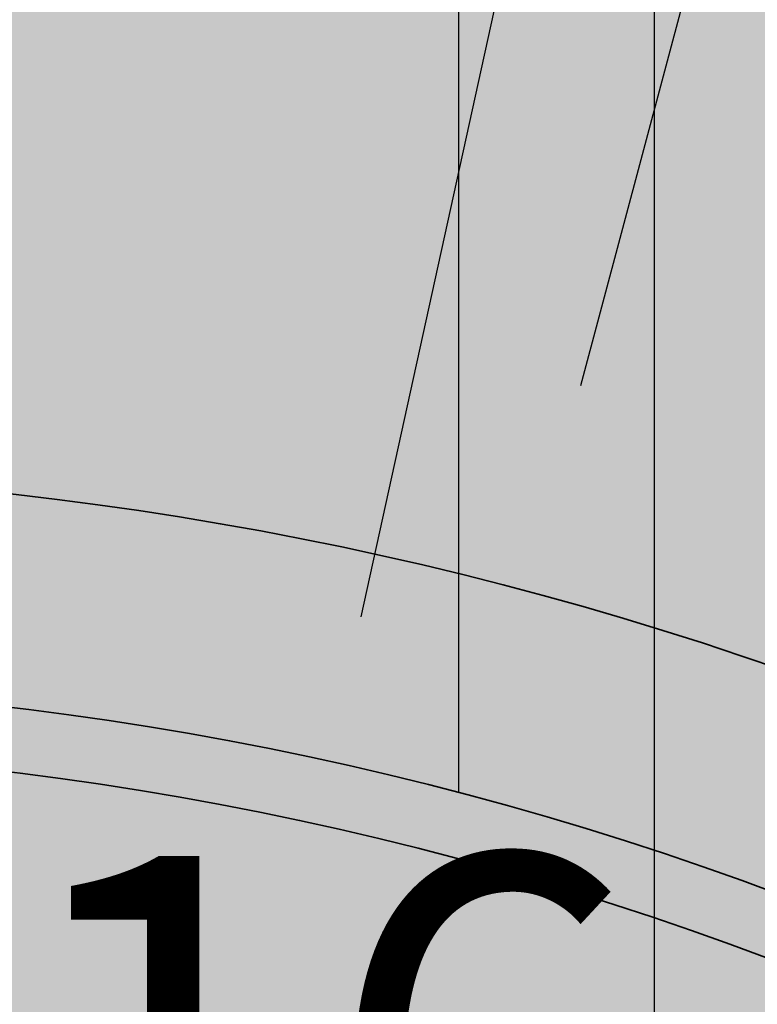
# Model space of a CAD drawing. Units: millimetres. Extents: x 130 to 1021, y 147 to 699.
# Tile 8 of 40: x 446 to 481, y 394 to 440. Entities that reach past the tile are written whole.
import ezdxf

# ---------------------------------------------------------------- set-up
doc = ezdxf.new("R2010")
doc.units = ezdxf.units.MM
doc.header["$MEASUREMENT"] = 0
for name, color, linetype, lineweight in [('A-ANNO-DIMS', 2, 'Continuous', 18), ('A-ELEV', 7, 'Continuous', 35), ('A-ELEV-PATT', 9, 'Continuous', 13)]:
    doc.layers.add(name, color=color, linetype=linetype, lineweight=lineweight)
doc.styles.get("Standard").update_dxf_attribs({"font": 'arial.ttf'})
doc.dimstyles.get("Standard").update_dxf_attribs({"dimtxt": 20, "dimasz": 10, "dimexe": 10, "dimexo": 10, "dimgap": 5, "dimtad": 0, "dimtih": 1, "dimtoh": 1, "dimdec": 0, "dimzin": 0, "dimdsep": 46, "dimtxsty": 'Standard', "dimcen": 5, "dimadec": 0, "dimazin": 0, "dimtfac": 1, "dimtdec": 0, "dimtofl": 0, "dimtmove": 0, "dimatfit": 3, "dimfxl": 1, "dimtolj": 1, "dimtzin": 0, "dimarcsym": 0})

# ---------------------------------------------------------------- blocks, each defined once
blk = doc.blocks.new('*D7')
at = {"layer": 'A-ANNO-DIMS', "color": 0, "lineweight": -2, "transparency": 16777216}
for p, q in [((399.374, 349.447), (413.374, 349.447)), ((423.374, 349.447), (433.374, 349.447)), ((389.374, 344.547), (389.374, 339.447)), ((423.374, 344.547), (423.374, 339.447))]:
    blk.add_line(p, q, dxfattribs=at)
at = {"layer": 'A-ANNO-DIMS', "color": 0, "transparency": 16777216}
for points in [[(399.374, 351.114), (399.374, 347.781), (389.374, 349.447)], [(413.374, 351.114), (413.374, 347.781), (423.374, 349.447)]]:
    blk.add_solid(points, dxfattribs=at)
at = {"layer": 'Defpoints', "color": 0, "transparency": 16777216}
for p in [(389.374, 354.547), (423.374, 354.547), (423.374, 349.447)]:
    blk.add_point(p, dxfattribs=at)
at = {"layer": 'A-ANNO-DIMS', "color": 0, "transparency": 16777216, "insert": (582.037, 349.447), "char_height": 20, "attachment_point": 5}
blk.add_mtext('\\A1;DOOR PANEL 34 TYP.', dxfattribs=at)
blk = doc.blocks.new('*D8')
at = {"layer": 'A-ANNO-DIMS', "color": 0, "lineweight": -2, "transparency": 16777216}
for p, q in [((428.474, 380.947), (428.474, 390.947)), ((428.474, 390.947), (438.474, 390.947)), ((433.374, 370.947), (438.474, 370.947)), ((433.374, 354.547), (438.474, 354.547)), ((428.474, 344.547), (428.474, 334.547))]:
    blk.add_line(p, q, dxfattribs=at)
at = {"layer": 'A-ANNO-DIMS', "color": 0, "transparency": 16777216}
for points in [[(426.807, 380.947), (430.14, 380.947), (428.474, 370.947)], [(426.807, 344.547), (430.14, 344.547), (428.474, 354.547)]]:
    blk.add_solid(points, dxfattribs=at)
at = {"layer": 'Defpoints', "color": 0, "transparency": 16777216}
for p in [(423.374, 370.947), (428.474, 370.947), (423.374, 354.547)]:
    blk.add_point(p, dxfattribs=at)
at = {"layer": 'A-ANNO-DIMS', "color": 0, "transparency": 16777216, "insert": (491.209, 390.947), "char_height": 20, "attachment_point": 5}
blk.add_mtext('\\A1;16 TYP.', dxfattribs=at)
blk = doc.blocks.new('*D11')
at = {"layer": 'A-ANNO-DIMS', "color": 0, "lineweight": -2, "transparency": 16777216}
for p, q in [((737.374, 648.699), (737.374, 149.739)), ((299.374, 566.947), (299.374, 149.739)), ((309.374, 159.739), (490.857, 159.739)), ((727.374, 159.739), (545.891, 159.739))]:
    blk.add_line(p, q, dxfattribs=at)
at = {"layer": 'A-ANNO-DIMS', "color": 0, "transparency": 16777216}
for points in [[(309.374, 161.406), (309.374, 158.073), (299.374, 159.739)], [(727.374, 161.406), (727.374, 158.073), (737.374, 159.739)]]:
    blk.add_solid(points, dxfattribs=at)
at = {"layer": 'Defpoints', "color": 0, "transparency": 16777216}
for p in [(737.374, 658.699), (299.374, 576.947), (737.374, 159.739)]:
    blk.add_point(p, dxfattribs=at)
at = {"layer": 'A-ANNO-DIMS', "color": 0, "transparency": 16777216, "insert": (518.374, 159.739), "char_height": 20, "attachment_point": 5}
blk.add_mtext('\\A1;438', dxfattribs=at)
blk = doc.blocks.new('*D12')
at = {"layer": 'A-ANNO-DIMS', "color": 0, "lineweight": -2, "transparency": 16777216}
for p, q in [((477.374, 661.947), (265.074, 661.947)), ((275.074, 651.947), (275.074, 438.205)), ((275.074, 194.039), (275.074, 407.782)), ((357.163, 184.039), (265.074, 184.039))]:
    blk.add_line(p, q, dxfattribs=at)
at = {"layer": 'A-ANNO-DIMS', "color": 0, "transparency": 16777216}
for points in [[(273.407, 651.947), (276.74, 651.947), (275.074, 661.947)], [(273.407, 194.039), (276.74, 194.039), (275.074, 184.039)]]:
    blk.add_solid(points, dxfattribs=at)
at = {"layer": 'Defpoints', "color": 0, "transparency": 16777216}
for p in [(275.074, 661.947), (487.374, 661.947), (367.163, 184.039)]:
    blk.add_point(p, dxfattribs=at)
at = {"layer": 'A-ANNO-DIMS', "color": 0, "transparency": 16777216, "insert": (275.074, 422.993), "char_height": 20, "attachment_point": 5}
blk.add_mtext('\\A1;477.9', dxfattribs=at)
blk = doc.blocks.new('*D16')
at = {"layer": 'A-ANNO-DIMS', "color": 0, "lineweight": -2, "transparency": 16777216}
for p, q in [((357.941, 411.947), (357.941, 696.247)), ((363.922, 579.884), (363.922, 696.247)), ((347.941, 686.247), (337.941, 686.247)), ((373.922, 686.247), (383.922, 686.247))]:
    blk.add_line(p, q, dxfattribs=at)
at = {"layer": 'A-ANNO-DIMS', "color": 0, "transparency": 16777216}
for points in [[(347.941, 687.914), (347.941, 684.581), (357.941, 686.247)], [(373.922, 687.914), (373.922, 684.581), (363.922, 686.247)]]:
    blk.add_solid(points, dxfattribs=at)
at = {"layer": 'Defpoints', "color": 0, "transparency": 16777216}
for p in [(363.922, 686.247), (363.922, 569.884), (357.941, 401.947)]:
    blk.add_point(p, dxfattribs=at)
at = {"layer": 'A-ANNO-DIMS', "color": 0, "transparency": 16777216, "insert": (420.737, 686.247), "char_height": 20, "attachment_point": 5}
blk.add_mtext('\\A1;5.981', dxfattribs=at)
blk = doc.blocks.new('*D18')
at = {"layer": 'A-ANNO-DIMS', "color": 0, "lineweight": -2, "transparency": 16777216}
for p, q in [((375.85, 490.216), (375.85, 696.247)), ((382.374, 388.947), (382.374, 696.247)), ((365.85, 686.247), (355.85, 686.247)), ((392.374, 686.247), (402.374, 686.247))]:
    blk.add_line(p, q, dxfattribs=at)
at = {"layer": 'A-ANNO-DIMS', "color": 0, "transparency": 16777216}
for points in [[(365.85, 687.914), (365.85, 684.581), (375.85, 686.247)], [(392.374, 687.914), (392.374, 684.581), (382.374, 686.247)]]:
    blk.add_solid(points, dxfattribs=at)
at = {"layer": 'Defpoints', "color": 0, "transparency": 16777216}
for p in [(382.374, 686.247), (375.85, 480.216), (382.374, 378.947)]:
    blk.add_point(p, dxfattribs=at)
at = {"layer": 'A-ANNO-DIMS', "color": 0, "transparency": 16777216, "insert": (441.132, 686.247), "char_height": 20, "attachment_point": 5}
blk.add_mtext('\\A1;6.524', dxfattribs=at)
blk = doc.blocks.new('*D19')
at = {"layer": 'A-ANNO-DIMS', "color": 0, "lineweight": -2, "transparency": 16777216}
for p, q in [((382.374, 388.947), (382.374, 696.247)), ((414.652, 510.881), (414.652, 696.247)), ((392.374, 686.247), (404.652, 686.247)), ((414.652, 686.247), (424.652, 686.247))]:
    blk.add_line(p, q, dxfattribs=at)
at = {"layer": 'A-ANNO-DIMS', "color": 0, "transparency": 16777216}
for points in [[(392.374, 687.914), (392.374, 684.581), (382.374, 686.247)], [(404.652, 687.914), (404.652, 684.581), (414.652, 686.247)]]:
    blk.add_solid(points, dxfattribs=at)
at = {"layer": 'Defpoints', "color": 0, "transparency": 16777216}
for p in [(414.652, 686.247), (414.652, 500.881), (382.374, 378.947)]:
    blk.add_point(p, dxfattribs=at)
at = {"layer": 'A-ANNO-DIMS', "color": 0, "transparency": 16777216, "insert": (463.411, 686.247), "char_height": 20, "attachment_point": 5}
blk.add_mtext('\\A1;32.28', dxfattribs=at)
blk = doc.blocks.new('*D20')
at = {"layer": 'A-ANNO-DIMS', "color": 0, "lineweight": -2, "transparency": 16777216}
for p, q in [((414.652, 510.881), (414.652, 696.247)), ((432.374, 388.947), (432.374, 696.247)), ((404.652, 686.247), (394.652, 686.247)), ((442.374, 686.247), (452.374, 686.247))]:
    blk.add_line(p, q, dxfattribs=at)
at = {"layer": 'A-ANNO-DIMS', "color": 0, "transparency": 16777216}
for points in [[(404.652, 687.914), (404.652, 684.581), (414.652, 686.247)], [(442.374, 687.914), (442.374, 684.581), (432.374, 686.247)]]:
    blk.add_solid(points, dxfattribs=at)
at = {"layer": 'Defpoints', "color": 0, "transparency": 16777216}
for p in [(432.374, 686.247), (414.652, 500.881), (432.374, 378.947)]:
    blk.add_point(p, dxfattribs=at)
at = {"layer": 'A-ANNO-DIMS', "color": 0, "transparency": 16777216, "insert": (490.075, 686.247), "char_height": 20, "attachment_point": 5}
blk.add_mtext('\\A1;17.72', dxfattribs=at)
blk = doc.blocks.new('*D21')
at = {"layer": 'A-ANNO-DIMS', "color": 0, "lineweight": -2, "transparency": 16777216}
for p, q in [((432.374, 388.947), (432.374, 696.247)), ((447.374, 656.947), (447.374, 696.247)), ((422.374, 686.247), (412.374, 686.247)), ((457.374, 686.247), (467.374, 686.247))]:
    blk.add_line(p, q, dxfattribs=at)
at = {"layer": 'A-ANNO-DIMS', "color": 0, "transparency": 16777216}
for points in [[(422.374, 687.914), (422.374, 684.581), (432.374, 686.247)], [(457.374, 687.914), (457.374, 684.581), (447.374, 686.247)]]:
    blk.add_solid(points, dxfattribs=at)
at = {"layer": 'Defpoints', "color": 0, "transparency": 16777216}
for p in [(447.374, 686.247), (447.374, 646.947), (432.374, 378.947)]:
    blk.add_point(p, dxfattribs=at)
at = {"layer": 'A-ANNO-DIMS', "color": 0, "transparency": 16777216, "insert": (485.832, 686.247), "char_height": 20, "attachment_point": 5}
blk.add_mtext('\\A1;15', dxfattribs=at)
blk = doc.blocks.new('*D22')
at = {"layer": 'A-ANNO-DIMS', "color": 0, "lineweight": -2, "transparency": 16777216}
for p, q in [((447.374, 656.947), (447.374, 696.247)), ((466.767, 403.947), (466.767, 696.247)), ((437.374, 686.247), (427.374, 686.247)), ((476.767, 686.247), (486.767, 686.247))]:
    blk.add_line(p, q, dxfattribs=at)
at = {"layer": 'A-ANNO-DIMS', "color": 0, "transparency": 16777216}
for points in [[(437.374, 687.914), (437.374, 684.581), (447.374, 686.247)], [(476.767, 687.914), (476.767, 684.581), (466.767, 686.247)]]:
    blk.add_solid(points, dxfattribs=at)
at = {"layer": 'Defpoints', "color": 0, "transparency": 16777216}
for p in [(466.767, 686.247), (447.374, 646.947), (466.767, 393.947)]:
    blk.add_point(p, dxfattribs=at)
at = {"layer": 'A-ANNO-DIMS', "color": 0, "transparency": 16777216, "insert": (532.34, 686.247), "char_height": 20, "attachment_point": 5}
blk.add_mtext('\\A1;19.393', dxfattribs=at)
blk = doc.blocks.new('*D23')
at = {"layer": 'A-ANNO-DIMS', "color": 0, "lineweight": -2, "transparency": 16777216}
for p, q in [((466.767, 403.947), (466.767, 696.247)), ((475.988, 209.039), (475.988, 696.247)), ((456.767, 686.247), (446.767, 686.247)), ((485.988, 686.247), (495.988, 686.247))]:
    blk.add_line(p, q, dxfattribs=at)
at = {"layer": 'A-ANNO-DIMS', "color": 0, "transparency": 16777216}
for points in [[(456.767, 687.914), (456.767, 684.581), (466.767, 686.247)], [(485.988, 687.914), (485.988, 684.581), (475.988, 686.247)]]:
    blk.add_solid(points, dxfattribs=at)
at = {"layer": 'Defpoints', "color": 0, "transparency": 16777216}
for p in [(475.988, 686.247), (466.767, 393.947), (475.988, 199.039)]:
    blk.add_point(p, dxfattribs=at)
at = {"layer": 'A-ANNO-DIMS', "color": 0, "transparency": 16777216, "insert": (534.631, 686.247), "char_height": 20, "attachment_point": 5}
blk.add_mtext('\\A1;9.222', dxfattribs=at)
blk = doc.blocks.new('*D24')
at = {"layer": 'A-ANNO-DIMS', "color": 0, "lineweight": -2, "transparency": 16777216}
for p, q in [((475.988, 209.039), (475.988, 696.247)), ((487.374, 671.947), (487.374, 696.247)), ((465.988, 686.247), (455.988, 686.247)), ((497.374, 686.247), (507.374, 686.247))]:
    blk.add_line(p, q, dxfattribs=at)
at = {"layer": 'A-ANNO-DIMS', "color": 0, "transparency": 16777216}
for points in [[(465.988, 687.914), (465.988, 684.581), (475.988, 686.247)], [(497.374, 687.914), (497.374, 684.581), (487.374, 686.247)]]:
    blk.add_solid(points, dxfattribs=at)
at = {"layer": 'Defpoints', "color": 0, "transparency": 16777216}
for p in [(487.374, 686.247), (487.374, 661.947), (475.988, 199.039)]:
    blk.add_point(p, dxfattribs=at)
at = {"layer": 'A-ANNO-DIMS', "color": 0, "transparency": 16777216, "insert": (553.022, 686.247), "char_height": 20, "attachment_point": 5}
blk.add_mtext('\\A1;11.385', dxfattribs=at)
blk = doc.blocks.new('*D64')
at = {"layer": 'A-ANNO-DIMS', "color": 0, "lineweight": -2, "transparency": 16777216}
for p, q in [((502.049, 450.926), (502.049, 460.926)), ((497.049, 455.926), (507.049, 455.926)), ((363.96, 263.061), (409.922, 327.255)), ((353.96, 263.061), (363.96, 263.061))]:
    blk.add_line(p, q, dxfattribs=at)
at = {"layer": 'A-ANNO-DIMS', "color": 0, "transparency": 16777216}
blk.add_solid([(408.567, 328.225), (411.277, 326.284), (415.743, 335.385)], dxfattribs=at)
at = {"layer": 'Defpoints', "color": 0, "transparency": 16777216}
for p in [(502.049, 455.926), (415.743, 335.385)]:
    blk.add_point(p, dxfattribs=at)
at = {"layer": 'A-ANNO-DIMS', "color": 0, "transparency": 16777216, "insert": (297.8, 263.061), "char_height": 20, "attachment_point": 5}
blk.add_mtext('\\A1;R148.25', dxfattribs=at)
blk = doc.blocks.new('*D65')
at = {"layer": 'A-ANNO-DIMS', "color": 0, "lineweight": -2, "transparency": 16777216}
for p, q in [((495.463, 509.127), (472.508, 423.108)), ((505.463, 509.127), (495.463, 509.127)), ((427.374, 248.979), (427.374, 258.979)), ((422.374, 253.979), (432.374, 253.979))]:
    blk.add_line(p, q, dxfattribs=at)
at = {"layer": 'A-ANNO-DIMS', "color": 0, "transparency": 16777216}
blk.add_solid([(470.898, 423.538), (474.118, 422.679), (469.93, 413.447)], dxfattribs=at)
at = {"layer": 'Defpoints', "color": 0, "transparency": 16777216}
for p in [(469.93, 413.447), (427.374, 253.979)]:
    blk.add_point(p, dxfattribs=at)
at = {"layer": 'A-ANNO-DIMS', "color": 0, "transparency": 16777216, "insert": (561.623, 509.127), "char_height": 20, "attachment_point": 5}
blk.add_mtext('\\A1;R165.05', dxfattribs=at)
blk = doc.blocks.new('*D67')
at = {"layer": 'A-ANNO-DIMS', "color": 0, "lineweight": -2, "transparency": 16777216}
for p, q in [((479.756, 492.431), (462.144, 412.223)), ((489.756, 492.431), (479.756, 492.431)), ((427.07, 247.496), (427.07, 257.496)), ((422.07, 252.496), (432.07, 252.496))]:
    blk.add_line(p, q, dxfattribs=at)
at = {"layer": 'A-ANNO-DIMS', "color": 0, "transparency": 16777216}
blk.add_solid([(460.516, 412.58), (463.772, 411.865), (459.999, 402.455)], dxfattribs=at)
at = {"layer": 'Defpoints', "color": 0, "transparency": 16777216}
for p in [(459.999, 402.455), (427.07, 252.496)]:
    blk.add_point(p, dxfattribs=at)
at = {"layer": 'A-ANNO-DIMS', "color": 0, "transparency": 16777216, "insert": (545.841, 492.431), "char_height": 20, "attachment_point": 5}
blk.add_mtext('\\A1;R153.53', dxfattribs=at)
blk = doc.blocks.new('*D69')
at = {"layer": 'A-ANNO-DIMS', "color": 0, "lineweight": -2, "transparency": 16777216}
for p, q in [((507.746, 572.261), (483.091, 501.813)), ((517.746, 572.261), (507.746, 572.261)), ((433.191, 354.23), (433.191, 364.23)), ((428.191, 359.23), (438.191, 359.23))]:
    blk.add_line(p, q, dxfattribs=at)
at = {"layer": 'A-ANNO-DIMS', "color": 0, "transparency": 16777216}
blk.add_solid([(481.518, 502.363), (484.664, 501.262), (479.788, 492.374)], dxfattribs=at)
at = {"layer": 'Defpoints', "color": 0, "transparency": 16777216}
for p in [(479.788, 492.374), (433.191, 359.23)]:
    blk.add_point(p, dxfattribs=at)
at = {"layer": 'A-ANNO-DIMS', "color": 0, "transparency": 16777216, "insert": (573.824, 572.261), "char_height": 20, "attachment_point": 5}
blk.add_mtext('\\A1;R141.06', dxfattribs=at)
blk = doc.blocks.new('*D71')
at = {"layer": 'A-ANNO-DIMS', "color": 0, "lineweight": -2, "transparency": 16777216}
for p, q in [((492.108, 581.609), (472.542, 512.666)), ((502.108, 581.609), (492.108, 581.609)), ((432.65, 367.109), (432.65, 377.109)), ((427.65, 372.109), (437.65, 372.109))]:
    blk.add_line(p, q, dxfattribs=at)
at = {"layer": 'A-ANNO-DIMS', "color": 0, "transparency": 16777216}
blk.add_solid([(470.938, 513.121), (474.145, 512.211), (469.812, 503.046)], dxfattribs=at)
at = {"layer": 'Defpoints', "color": 0, "transparency": 16777216}
for p in [(469.812, 503.046), (432.65, 372.109)]:
    blk.add_point(p, dxfattribs=at)
at = {"layer": 'A-ANNO-DIMS', "color": 0, "transparency": 16777216, "insert": (548.493, 581.609), "char_height": 20, "attachment_point": 5}
blk.add_mtext('\\A1;R136.1', dxfattribs=at)
blk = doc.blocks.new('*D72')
at = {"layer": 'A-ANNO-DIMS', "color": 0, "lineweight": -2, "transparency": 16777216}
for p, q in [((460.658, 573.64), (451.279, 503.49)), ((470.658, 573.64), (460.658, 573.64)), ((432.115, 355.142), (432.115, 365.142)), ((427.115, 360.142), (437.115, 360.142))]:
    blk.add_line(p, q, dxfattribs=at)
at = {"layer": 'A-ANNO-DIMS', "color": 0, "transparency": 16777216}
blk.add_solid([(449.628, 503.711), (452.931, 503.27), (449.954, 493.579)], dxfattribs=at)
at = {"layer": 'Defpoints', "color": 0, "transparency": 16777216}
for p in [(449.954, 493.579), (432.115, 360.142)]:
    blk.add_point(p, dxfattribs=at)
at = {"layer": 'A-ANNO-DIMS', "color": 0, "transparency": 16777216, "insert": (526.64, 573.64), "char_height": 20, "attachment_point": 5}
blk.add_mtext('\\A1;R134.62', dxfattribs=at)

msp = doc.modelspace()

# ---------------------------------------------------------------- hatches: boundary and pattern name
at = {"layer": 'A-ELEV-PATT'}
h = msp.add_hatch(color=256, dxfattribs=at)
h.dxf.hatch_style = 1
h.paths.add_polyline_path([(737.3738, 658.6988, 0.0135961), (632.4019, 661.9473), (607.3738, 661.9473), (487.3738, 661.9473), (487.3738, 649.9473), (607.3738, 649.9473), (632.3794, 649.9473, -0.0136841), (737.3738, 646.6784)])
h.paths.add_polyline_path([(732.3738, 643.9599, 0.0130529), (632.3738, 646.9473), (607.3738, 646.9473), (487.3738, 646.9473), (487.3738, 596.9473), (632.3738, 596.9473, -0.0130529), (732.3738, 593.9599)])
h.paths.add_polyline_path([(737.3738, 593.6732, 0.0137063), (632.3738, 596.9473), (487.3738, 596.9473), (487.3738, 586.9473), (632.355, 586.9473, -0.0137808), (737.3738, 583.6559)])
h.paths.add_polyline_path([(447.3738, 646.9473), (307.3738, 646.9473), (302.3738, 646.9473), (302.3738, 634.9473), (447.3738, 634.9473)])
h.paths.add_polyline_path([(447.3738, 631.9473), (307.3738, 631.9473), (307.3738, 586.9473), (447.3738, 586.9473)])
h.paths.add_polyline_path([(447.3738, 586.9473), (307.3738, 586.9473), (302.3738, 586.9473), (302.3738, 576.9473), (447.3738, 576.9473)])
h.paths.add_polyline_path([(447.3738, 573.9473), (367.3738, 573.9473), (367.3738, 539.9473), (447.3738, 539.9473)])
h.paths.add_polyline_path([(447.3738, 537.9473), (367.3738, 537.9473), (367.3738, 507.9473), (400.392, 507.4253, -0.001728), (401.3281, 507.6451, -0.5220025), (425.6117, 511.0391, -0.0391849), (447.3738, 510.4359), (447.3738, 510.7883)])
h.paths.add_polyline_path([(394.7238, 505.9473), (367.3738, 505.9473), (367.3738, 476.9473, -0.0146512), (375.8501, 480.2159), (376.1506, 499.2266, -0.0355419)])
h.paths.add_polyline_path([(632.3738, 583.9473), (552.3738, 583.9473), (552.3738, 550.9473), (632.3738, 550.9473)])
h.paths.add_polyline_path([(632.3738, 548.9473), (552.3738, 548.9473), (552.3738, 515.9473), (632.3738, 515.9473)])
h.paths.add_polyline_path([(632.3738, 513.9473), (552.3738, 513.9473), (552.3738, 476.9473), (632.3738, 476.9473)])
h.paths.add_polyline_path([(737.3738, 473.6903, 0.0136326), (632.3926, 476.9473), (552.3738, 476.9473), (487.3738, 476.9473), (487.3738, 466.9473), (632.3738, 466.9473, -0.0137063), (737.3738, 463.6732)])
h.paths.add_polyline_path([(732.3738, 460.9552, 0.0130741), (632.3681, 463.9473), (487.3738, 463.9473), (487.3738, 407.735, -0.0032286), (489.3544, 406.9473), (632.3926, 406.9473, -0.0129826), (732.3738, 403.9755)])
h.paths.add_polyline_path([(487.3738, 463.9473, 0.20133), (367.3738, 463.9473), (367.3738, 407.735, -0.1882031), (487.3738, 407.735)])
h.paths.add_polyline_path([(367.3738, 476.9473), (367.3738, 466.9473, -0.2013309), (487.3738, 466.9473), (487.3738, 476.9473, 0.20133)])
h.paths.add_polyline_path([(367.3738, 463.9473), (307.3738, 463.9473), (307.3738, 401.9473), (357.9413, 401.9473), (367.3738, 407.735)])
h.paths.add_polyline_path([(367.3738, 476.9473), (302.3738, 476.9473), (302.3738, 466.9473), (367.3738, 466.9473)])
h.paths.add_polyline_path([(632.8184, 366.9453), (552.3738, 366.9453), (552.3738, 393.9473), (632.8184, 393.9473)])
h.paths.add_polyline_path([(632.8184, 357.2114), (632.8184, 363.9453), (552.3738, 363.9453), (552.3738, 357.2114), (552.3738, 336.9453), (632.8184, 336.9453)])
h.paths.add_polyline_path([(632.8184, 333.9453), (552.3738, 333.9453), (552.3738, 306.9453), (632.8184, 306.9453)])
h.paths.add_polyline_path([(632.8184, 303.9453), (552.3738, 303.9453), (552.3738, 273.9473), (632.355, 273.9473, 0.0000608), (632.8184, 273.9491)])
h.paths.add_polyline_path([(737.3738, 403.6903, 0.0136326), (632.3926, 406.9473), (489.3544, 406.9473, 0.1915481), (367.3738, 407.735), (367.3738, 396.9473, -0.2013309), (487.3738, 396.9473), (632.3738, 396.9473, -0.0137063), (737.3738, 393.6732)])
h.paths.add_polyline_path([(357.9413, 401.9473), (307.3738, 401.9473), (307.3738, 391.9473), (357.9413, 391.9473)])
h.paths.add_polyline_path([(357.9413, 357.2114), (357.9413, 388.9473), (307.3738, 388.9473), (307.3738, 357.2114), (307.3738, 273.9473), (357.9413, 273.9473)])
h.paths.add_polyline_path([(732.3738, 263.93, -0.0130317), (632.3794, 260.9473), (466.7667, 260.9473), (466.7667, 240.9473), (469.8406, 236.978), (469.8406, 221.978), (472.9145, 218.0087), (472.9145, 213.9473), (607.3738, 213.9473), (732.3738, 213.9473)])
h.paths.add_polyline_path([(732.3738, 290.889), (722.479, 290.889), (722.479, 301.889), (732.3738, 301.889), (732.3738, 305.889), (722.479, 305.889), (722.479, 316.889), (732.3738, 316.889), (732.3738, 320.889), (722.479, 320.889), (722.479, 331.889), (732.3738, 331.889), (732.3738, 335.889), (722.479, 335.889), (722.479, 346.889), (732.3738, 346.889), (732.3738, 350.889), (722.479, 350.889), (722.479, 361.889), (732.3738, 361.889), (732.3738, 365.889), (722.479, 365.889), (722.479, 376.889), (732.3738, 376.889), (732.3738, 380.889), (722.479, 380.889), (722.479, 391.4848, 0.0005233), (718.479, 391.6843), (718.479, 380.889), (707.479, 380.889), (707.479, 392.1896, 0.0005231), (703.479, 392.3576), (703.479, 380.889), (692.479, 380.889), (692.479, 392.7765, 0.0005229), (688.479, 392.9131), (688.479, 380.889), (677.479, 380.889), (677.479, 393.2456, 0.0005228), (673.479, 393.3508), (673.479, 380.889), (662.479, 380.889), (662.479, 393.597, 0.0005227), (658.479, 393.6709), (658.479, 380.889), (647.479, 380.889), (647.479, 393.8308, 0.0005226), (643.479, 393.8732), (643.479, 380.889), (632.8184, 380.889), (632.8184, 376.889), (643.479, 376.889), (643.479, 365.889), (632.8184, 365.889), (632.8184, 361.889), (643.479, 361.889), (643.479, 350.889), (632.8184, 350.889), (632.8184, 346.889), (643.479, 346.889), (643.479, 335.889), (632.8184, 335.889), (632.8184, 331.889), (643.479, 331.889), (643.479, 320.889), (632.8184, 320.889), (632.8184, 316.889), (643.479, 316.889), (643.479, 305.889), (632.8184, 305.889), (632.8184, 301.889), (643.479, 301.889), (643.479, 290.889), (632.8184, 290.889), (632.8184, 286.889), (643.479, 286.889), (643.479, 274.0217, 0.0005246), (647.479, 274.0643), (647.479, 286.889), (658.479, 286.889), (658.479, 274.2248, 0.0005246), (662.479, 274.2989), (662.479, 286.889), (673.479, 286.889), (673.479, 274.546, 0.0005247), (677.479, 274.6516), (677.479, 286.889), (688.479, 286.889), (688.479, 274.9853, 0.0005248), (692.479, 275.1224), (692.479, 286.889), (703.479, 286.889), (703.479, 275.5429, 0.000525), (707.479, 275.7115), (707.479, 286.889), (718.479, 286.889), (718.479, 276.2187, 0.0005252), (722.479, 276.4189), (722.479, 286.889), (732.3738, 286.889)])
h.paths.add_polyline_path([(718.479, 290.889), (707.479, 290.889), (707.479, 301.889), (718.479, 301.889)], flags=16)
h.paths.add_polyline_path([(703.479, 290.889), (692.479, 290.889), (692.479, 301.889), (703.479, 301.889)], flags=16)
h.paths.add_polyline_path([(718.479, 305.889), (707.479, 305.889), (707.479, 316.889), (718.479, 316.889)], flags=16)
h.paths.add_polyline_path([(703.479, 305.889), (692.479, 305.889), (692.479, 316.889), (703.479, 316.889)], flags=16)
h.paths.add_polyline_path([(688.479, 290.889), (677.479, 290.889), (677.479, 301.889), (688.479, 301.889)], flags=16)
h.paths.add_polyline_path([(718.479, 320.889), (707.479, 320.889), (707.479, 331.889), (718.479, 331.889)], flags=16)
h.paths.add_polyline_path([(688.479, 305.889), (677.479, 305.889), (677.479, 316.889), (688.479, 316.889)], flags=16)
h.paths.add_polyline_path([(703.479, 320.889), (692.479, 320.889), (692.479, 331.889), (703.479, 331.889)], flags=16)
h.paths.add_polyline_path([(688.479, 320.889), (677.479, 320.889), (677.479, 331.889), (688.479, 331.889)], flags=16)
h.paths.add_polyline_path([(673.479, 290.889), (662.479, 290.889), (662.479, 301.889), (673.479, 301.889)], flags=16)
h.paths.add_polyline_path([(718.479, 335.889), (707.479, 335.889), (707.479, 346.889), (718.479, 346.889)], flags=16)
h.paths.add_polyline_path([(673.479, 305.889), (662.479, 305.889), (662.479, 316.889), (673.479, 316.889)], flags=16)
h.paths.add_polyline_path([(703.479, 335.889), (692.479, 335.889), (692.479, 346.889), (703.479, 346.889)], flags=16)
h.paths.add_polyline_path([(673.479, 320.889), (662.479, 320.889), (662.479, 331.889), (673.479, 331.889)], flags=16)
h.paths.add_polyline_path([(688.479, 335.889), (677.479, 335.889), (677.479, 346.889), (688.479, 346.889)], flags=16)
h.paths.add_polyline_path([(658.479, 290.889), (647.479, 290.889), (647.479, 301.889), (658.479, 301.889)], flags=16)
h.paths.add_polyline_path([(718.479, 350.889), (707.479, 350.889), (707.479, 361.889), (718.479, 361.889)], flags=16)
h.paths.add_polyline_path([(658.479, 305.889), (647.479, 305.889), (647.479, 316.889), (658.479, 316.889)], flags=16)
h.paths.add_polyline_path([(703.479, 350.889), (692.479, 350.889), (692.479, 361.889), (703.479, 361.889)], flags=16)
h.paths.add_polyline_path([(673.479, 335.889), (662.479, 335.889), (662.479, 346.889), (673.479, 346.889)], flags=16)
h.paths.add_polyline_path([(658.479, 320.889), (647.479, 320.889), (647.479, 331.889), (658.479, 331.889)], flags=16)
h.paths.add_polyline_path([(688.479, 350.889), (677.479, 350.889), (677.479, 361.889), (688.479, 361.889)], flags=16)
h.paths.add_polyline_path([(718.479, 365.889), (707.479, 365.889), (707.479, 376.889), (718.479, 376.889)], flags=16)
h.paths.add_polyline_path([(658.479, 335.889), (647.479, 335.889), (647.479, 346.889), (658.479, 346.889)], flags=16)
h.paths.add_polyline_path([(673.479, 350.889), (662.479, 350.889), (662.479, 361.889), (673.479, 361.889)], flags=16)
h.paths.add_polyline_path([(703.479, 365.889), (692.479, 365.889), (692.479, 376.889), (703.479, 376.889)], flags=16)
h.paths.add_polyline_path([(688.479, 365.889), (677.479, 365.889), (677.479, 376.889), (688.479, 376.889)], flags=16)
h.paths.add_polyline_path([(658.479, 350.889), (647.479, 350.889), (647.479, 361.889), (658.479, 361.889)], flags=16)
h.paths.add_polyline_path([(673.479, 365.889), (662.479, 365.889), (662.479, 376.889), (673.479, 376.889)], flags=16)
h.paths.add_polyline_path([(658.479, 365.889), (647.479, 365.889), (647.479, 376.889), (658.479, 376.889)], flags=16)
h.paths.add_polyline_path([(732.3738, 503.9786), (722.3392, 503.9786), (722.3392, 514.9786), (732.3738, 514.9786), (732.3738, 518.9786), (722.3392, 518.9786), (722.3392, 529.9786), (732.3738, 529.9786), (732.3738, 533.9786), (722.3392, 533.9786), (722.3392, 544.9786), (732.3738, 544.9786), (732.3738, 546.9473), (732.3738, 548.9786), (722.3392, 548.9786), (722.3392, 559.9786), (732.3738, 559.9786), (732.3738, 563.9786), (722.3392, 563.9786), (722.3392, 574.9786), (732.3738, 574.9786), (732.3738, 578.9786), (722.3392, 578.9786), (722.3392, 581.4789, 0.000526), (718.3392, 581.6791), (718.3392, 578.9786), (707.3392, 578.9786), (707.3392, 582.1863, 0.0005258), (703.3392, 582.355), (703.3392, 578.9786), (692.3392, 578.9786), (692.3392, 582.7752, 0.0005257), (688.3392, 582.9123), (688.3392, 578.9786), (677.3392, 578.9786), (677.3392, 583.2457, 0.0005255), (673.3392, 583.3512), (673.3392, 578.9786), (662.3392, 578.9786), (662.3392, 583.5978, 0.0005254), (658.3392, 583.6718), (658.3392, 578.9786), (647.3392, 578.9786), (647.3392, 583.8317, 0.0005254), (643.3392, 583.8741), (643.3392, 578.9786), (632.3738, 578.9786), (632.3738, 574.9786), (643.3392, 574.9786), (643.3392, 563.9786), (632.3738, 563.9786), (632.3738, 559.9786), (643.3392, 559.9786), (643.3392, 548.9786), (632.3738, 548.9786), (632.3738, 544.9786), (643.3392, 544.9786), (643.3392, 533.9786), (632.3738, 533.9786), (632.3738, 529.9786), (643.3392, 529.9786), (643.3392, 518.9786), (632.3738, 518.9786), (632.3738, 515.9473), (632.3738, 514.9786), (643.3392, 514.9786), (643.3392, 503.9786), (632.3738, 503.9786), (632.3738, 499.9786), (643.3392, 499.9786), (643.3392, 488.9786), (632.3738, 488.9786), (632.3738, 484.9786), (643.3392, 484.9786), (643.3392, 476.8751, -0.0005191), (647.3392, 476.8332), (647.3392, 484.9786), (658.3392, 484.9786), (658.3392, 476.6752, -0.0005192), (662.3392, 476.6022), (662.3392, 484.9786), (673.3392, 484.9786), (673.3392, 476.3585, -0.0005193), (677.3392, 476.2543), (677.3392, 484.9786), (688.3392, 484.9786), (688.3392, 475.9248, -0.0005194), (692.3392, 475.7894), (692.3392, 484.9786), (703.3392, 484.9786), (703.3392, 475.3741, -0.0005195), (707.3392, 475.2075), (707.3392, 484.9786), (718.3392, 484.9786), (718.3392, 474.7064, -0.0005197), (722.3392, 474.5086), (722.3392, 484.9786), (732.3738, 484.9786), (732.3738, 488.9786), (722.3392, 488.9786), (722.3392, 499.9786), (732.3738, 499.9786)])
h.paths.add_polyline_path([(718.3392, 503.9786), (707.3392, 503.9786), (707.3392, 514.9786), (718.3392, 514.9786)], flags=16)
h.paths.add_polyline_path([(718.3392, 499.9786), (718.3392, 488.9786), (707.3392, 488.9786), (707.3392, 499.9786)], flags=16)
h.paths.add_polyline_path([(718.3392, 518.9786), (707.3392, 518.9786), (707.3392, 529.9786), (718.3392, 529.9786)], flags=16)
h.paths.add_polyline_path([(703.3392, 503.9786), (692.3392, 503.9786), (692.3392, 514.9786), (703.3392, 514.9786)], flags=16)
h.paths.add_polyline_path([(703.3392, 499.9786), (703.3392, 488.9786), (692.3392, 488.9786), (692.3392, 499.9786)], flags=16)
h.paths.add_polyline_path([(703.3392, 518.9786), (692.3392, 518.9786), (692.3392, 529.9786), (703.3392, 529.9786)], flags=16)
h.paths.add_polyline_path([(718.3392, 533.9786), (707.3392, 533.9786), (707.3392, 544.9786), (718.3392, 544.9786)], flags=16)
h.paths.add_polyline_path([(688.3392, 503.9786), (677.3392, 503.9786), (677.3392, 514.9786), (688.3392, 514.9786)], flags=16)
h.paths.add_polyline_path([(688.3392, 499.9786), (688.3392, 488.9786), (677.3392, 488.9786), (677.3392, 499.9786)], flags=16)
h.paths.add_polyline_path([(703.3392, 533.9786), (692.3392, 533.9786), (692.3392, 544.9786), (703.3392, 544.9786)], flags=16)
h.paths.add_polyline_path([(688.3392, 518.9786), (677.3392, 518.9786), (677.3392, 529.9786), (688.3392, 529.9786)], flags=16)
h.paths.add_polyline_path([(688.3392, 533.9786), (677.3392, 533.9786), (677.3392, 544.9786), (688.3392, 544.9786)], flags=16)
h.paths.add_polyline_path([(718.3392, 548.9786), (707.3392, 548.9786), (707.3392, 559.9786), (718.3392, 559.9786)], flags=16)
h.paths.add_polyline_path([(673.3392, 503.9786), (662.3392, 503.9786), (662.3392, 514.9786), (673.3392, 514.9786)], flags=16)
h.paths.add_polyline_path([(673.3392, 499.9786), (673.3392, 488.9786), (662.3392, 488.9786), (662.3392, 499.9786)], flags=16)
h.paths.add_polyline_path([(703.3392, 548.9786), (692.3392, 548.9786), (692.3392, 559.9786), (703.3392, 559.9786)], flags=16)
h.paths.add_polyline_path([(673.3392, 518.9786), (662.3392, 518.9786), (662.3392, 529.9786), (673.3392, 529.9786)], flags=16)
h.paths.add_polyline_path([(688.3392, 548.9786), (677.3392, 548.9786), (677.3392, 559.9786), (688.3392, 559.9786)], flags=16)
h.paths.add_polyline_path([(673.3392, 533.9786), (662.3392, 533.9786), (662.3392, 544.9786), (673.3392, 544.9786)], flags=16)
h.paths.add_polyline_path([(718.3392, 563.9786), (707.3392, 563.9786), (707.3392, 574.9786), (718.3392, 574.9786)], flags=16)
h.paths.add_polyline_path([(658.3392, 503.9786), (647.3392, 503.9786), (647.3392, 514.9786), (658.3392, 514.9786)], flags=16)
h.paths.add_polyline_path([(658.3392, 499.9786), (658.3392, 488.9786), (647.3392, 488.9786), (647.3392, 499.9786)], flags=16)
h.paths.add_polyline_path([(703.3392, 563.9786), (692.3392, 563.9786), (692.3392, 574.9786), (703.3392, 574.9786)], flags=16)
h.paths.add_polyline_path([(658.3392, 518.9786), (647.3392, 518.9786), (647.3392, 529.9786), (658.3392, 529.9786)], flags=16)
h.paths.add_polyline_path([(673.3392, 548.9786), (662.3392, 548.9786), (662.3392, 559.9786), (673.3392, 559.9786)], flags=16)
h.paths.add_polyline_path([(688.3392, 563.9786), (677.3392, 563.9786), (677.3392, 574.9786), (688.3392, 574.9786)], flags=16)
h.paths.add_polyline_path([(658.3392, 533.9786), (647.3392, 533.9786), (647.3392, 544.9786), (658.3392, 544.9786)], flags=16)
h.paths.add_polyline_path([(673.3392, 563.9786), (662.3392, 563.9786), (662.3392, 574.9786), (673.3392, 574.9786)], flags=16)
h.paths.add_polyline_path([(658.3392, 548.9786), (647.3392, 548.9786), (647.3392, 559.9786), (658.3392, 559.9786)], flags=16)
h.paths.add_polyline_path([(658.3392, 563.9786), (647.3392, 563.9786), (647.3392, 574.9786), (658.3392, 574.9786)], flags=16)
h = msp.add_hatch(color=256, dxfattribs=at)
h.dxf.hatch_style = 1
h.paths.add_polyline_path([(447.3738, 576.9473), (302.3738, 576.9473), (302.3738, 573.9473), (447.3738, 573.9473)])
h.paths.add_polyline_path([(487.3738, 583.9473), (487.3738, 586.9473), (447.3738, 576.9473), (447.3738, 573.9473)])
h.paths.add_polyline_path([(632.355, 586.9473), (487.3738, 586.9473), (487.3738, 583.9473), (632.3738, 583.9473), (632.3738, 583.9472, -0.0138), (737.3738, 580.6507), (737.3738, 583.6559, 0.0137808)])
h.paths.add_polyline_path([(367.3738, 466.9473), (302.3738, 466.9473), (302.3738, 463.9473), (367.3738, 463.9473)])
h.paths.add_polyline_path([(487.3738, 463.9473), (487.3738, 466.9473, 0.2013309), (367.3738, 466.9473), (367.3738, 463.9473, -0.20133)])
h.paths.add_polyline_path([(632.3738, 466.9473), (487.3738, 466.9473), (487.3738, 463.9473), (632.3681, 463.9473, -0.0137285), (737.3738, 460.6681), (737.3738, 463.6732, 0.0137063)])
h.paths.add_polyline_path([(632.3738, 396.9473), (487.3738, 396.9473, 0.2013309), (367.3738, 396.9473), (367.3738, 393.9473, -0.2023717), (486.7667, 393.9473), (632.3681, 393.9473, -0.0137285), (737.3738, 390.6681), (737.3738, 393.6732, 0.0137063)])
h.paths.add_polyline_path([(357.9413, 391.9473), (307.3738, 391.9473), (307.3738, 388.9473), (357.9413, 388.9473)])
h.paths.add_polyline_path([(367.3738, 393.9473), (367.3738, 396.9473), (357.9413, 391.924), (357.9413, 388.9473), (358.058, 388.9473)])
h.paths.add_polyline_path([(737.3738, 264.2162), (737.3738, 267.2214, -0.0137063), (632.3738, 263.9473), (463.7667, 263.9473), (466.7667, 260.9473), (632.3794, 260.9473, 0.0136841)])
h.paths.add_polyline_path([(463.7667, 263.9473), (447.3738, 263.9473), (450.3738, 260.9473), (466.7667, 260.9473)])
h.paths.add_polyline_path([(447.3738, 263.9473), (432.3738, 263.9473), (432.3738, 260.9473), (450.3738, 260.9473)])
h.paths.add_polyline_path([(382.3738, 263.9473), (357.9413, 263.9473), (357.9413, 260.9473), (382.3738, 260.9473)])
h.paths.add_polyline_path([(357.9413, 263.9473), (307.3738, 263.9473), (307.3738, 260.9473), (357.9413, 260.9473)])
h = msp.add_hatch(color=256, dxfattribs=at)
h.paths.add_polyline_path([(327.3738, 569.884), (327.3738, 573.9473), (307.3738, 573.9473), (307.3738, 476.9473), (327.3738, 476.9473), (327.3738, 480.95)])
h.paths.add_polyline_path([(486.7667, 386.2639), (486.7667, 393.9473), (466.7667, 393.9473), (466.7667, 357.2114), (466.7667, 311.9335, 0.0342703), (486.7667, 308.4637)])
h.paths.add_polyline_path([(486.7667, 308.4637, -0.0342703), (466.7667, 311.9335), (466.7667, 273.9473), (486.7667, 273.9473)])
h.paths.add_polyline_path([(389.3738, 351.5473), (396.7693, 351.5473, -0.007027), (393.8774, 354.5473), (389.3738, 354.5473), (389.3738, 359.5775, -0.0190302), (382.3738, 368.424), (382.3738, 249.5473), (432.3738, 249.5473), (432.3738, 325.067, -0.0057673), (429.3738, 326.709), (429.3738, 257.5473), (426.3738, 257.5473), (426.3738, 328.4428, -0.0059254), (423.3738, 330.272), (423.3738, 315.7473), (389.3738, 315.7473), (389.3738, 332.1473), (420.4552, 332.1473, -0.008951), (416.0768, 335.1473), (389.3738, 335.1473)])
h.paths.add_polyline_path([(389.3738, 312.7473), (423.3738, 312.7473), (423.3738, 296.3473), (389.3738, 296.3473)], flags=16)
h.paths.add_polyline_path([(389.3738, 293.3473), (423.3738, 293.3473), (423.3738, 276.9473), (389.3738, 276.9473)], flags=16)
h.paths.add_polyline_path([(389.3738, 273.9473), (423.3738, 273.9473), (423.3738, 257.5473), (389.3738, 257.5473)], flags=16)
h.paths.add_polyline_path([(432.3738, 378.9473), (382.3738, 378.9473), (382.3738, 368.424, 0.0190302), (389.3738, 359.5775), (389.3738, 370.9473), (423.3738, 370.9473), (423.3738, 354.5473), (393.8774, 354.5473, 0.007027), (396.7693, 351.5473), (423.3738, 351.5473), (423.3738, 335.1473), (416.0768, 335.1473, 0.008951), (420.4552, 332.1473), (423.3738, 332.1473), (423.3738, 330.272, 0.0059254), (426.3738, 328.4428), (426.3738, 370.9473), (429.3738, 370.9473), (429.3738, 326.709, 0.0057673), (432.3738, 325.067)])
h.paths.add_polyline_path([(466.7667, 357.2114), (466.7667, 393.9473), (447.3738, 393.9473), (447.3738, 357.2114), (447.3738, 318.1243, 0.0063261), (450.8779, 316.785), (450.8779, 331.5915), (463.5608, 331.5915), (463.5608, 312.7571, 0.005582), (466.7667, 311.9335)])
h.paths.add_polyline_path([(450.8779, 334.5915), (450.8779, 360.0915), (463.5608, 360.0915), (463.5608, 334.5915)], flags=16)
h.paths.add_polyline_path([(450.8779, 363.0915), (450.8779, 388.6449), (463.5608, 388.6449), (463.5608, 363.0915)], flags=16)
h.paths.add_polyline_path([(466.7667, 311.9335, -0.005582), (463.5608, 312.7571), (463.5608, 306.0915), (450.8779, 306.0915), (450.8779, 316.785, -0.0063261), (447.3738, 318.1243), (447.3738, 273.9473), (466.7667, 273.9473)])
h.paths.add_polyline_path([(450.8779, 303.0915), (463.5608, 303.0915), (463.5608, 277.5915), (450.8779, 277.5915)], flags=16)
h.paths.add_polyline_path([(552.3738, 357.2114), (552.3738, 393.9473), (486.7667, 393.9473), (486.7667, 386.2639), (544.6354, 386.2639), (544.6354, 280.6619), (486.7667, 280.6619), (486.7667, 273.9473), (552.3738, 273.9473)])
h.paths.add_polyline_path([(487.3738, 583.9473), (472.3738, 580.1973), (472.3738, 507.0765), (472.3738, 505.4251, -0.0056452), (475.3738, 504.4942), (475.3738, 506.3543), (475.3738, 511.9473), (484.3738, 511.9473), (484.3738, 503.8134), (484.3738, 501.2439, -0.0058357), (487.3738, 500.0015)])
h.paths.add_polyline_path([(484.3738, 578.0434), (484.3738, 548.9473), (475.3738, 548.9473), (475.3738, 575.7934)], flags=16)
h.paths.add_polyline_path([(484.3738, 546.9473), (484.3738, 513.9473), (475.3738, 513.9473), (475.3738, 518.7148), (475.3738, 546.9473)], flags=16)
h = msp.add_hatch(color=256, dxfattribs=at)
h.dxf.hatch_style = 1
h.paths.add_polyline_path([(363.922, 569.884), (327.3738, 569.884), (327.3738, 557.9168), (363.922, 557.9168)])
h.paths.add_polyline_path([(547.7773, 577.3739), (502.3738, 577.3739), (502.3738, 566.2111), (547.7773, 566.2111)])
h.paths.add_polyline_path([(544.6354, 386.2639), (486.7667, 386.2639), (486.7667, 377.43), (544.6354, 377.43)])
h.paths.add_polyline_path([(496.0546, 377.43), (486.7667, 377.43), (486.7667, 370.4028)])
h.paths.add_polyline_path([(447.3738, 393.9473), (367.3738, 393.9473, 0.0500478), (382.3738, 368.424), (382.3738, 378.9473), (432.3738, 378.9473), (432.3738, 325.067, 0.0278945), (447.3738, 318.1243), (447.3738, 357.2114)])
h.paths.add_polyline_path([(463.5608, 388.6449), (450.8779, 388.6449), (450.8779, 363.0915), (463.5608, 363.0915)])
h.paths.add_polyline_path([(463.5608, 360.0915), (450.8779, 360.0915), (450.8779, 334.5915), (463.5608, 334.5915)])
h.paths.add_polyline_path([(463.5608, 331.5915), (450.8779, 331.5915), (450.8779, 316.785, 0.0224513), (463.5608, 312.7571)])
msp.add_hatch(color=256, dxfattribs=at).paths.add_polyline_path([(367.3738, 393.9473), (486.7667, 393.9473, 0.2023717)])

# ---------------------------------------------------------------- linework, layer by layer
at = {"layer": 'A-ELEV'}
for centre, radius, start, end in [((427.3738, 253.9788), 165.0484, 67.942927, 111.31713), ((427.3738, 253.9788), 155.0484, 67.233534, 112.766466), ((427.0702, 252.4956), 153.5326, 67.118929, 112.881071)]:
    msp.add_arc(centre, radius, start, end, dxfattribs=at)

# ---------------------------------------------------------------- dimensions: what is measured, and where the dimension line sits
at = {"layer": 'A-ANNO-DIMS'}
for base, p1, p2, override, picture, middle in [((363.922, 686.2473), (357.9413, 401.9473), (363.922, 569.884), {"dimdec": 3, "dimlfac": 1, "dimrnd": 0, "dimzin": 0, "dimdsep": 46, "dimlunit": 2}, '*D16', (420.7365, 686.2473)), ((382.3738, 686.2473), (375.8501, 480.2159), (382.3738, 378.9473), {"dimdec": 3, "dimlfac": 1, "dimrnd": 0, "dimzin": 0, "dimdsep": 46, "dimlunit": 2}, '*D18', (441.1323, 686.2473)), ((414.6525, 686.2473), (382.3738, 378.9473), (414.6525, 500.8811), {"dimdec": 2, "dimlfac": 1, "dimrnd": 0, "dimzin": 0, "dimdsep": 46, "dimlunit": 2}, '*D19', (463.411, 686.2473)), ((432.3738, 686.2473), (414.6525, 500.8811), (432.3738, 378.9473), {"dimdec": 2, "dimlfac": 1, "dimrnd": 0, "dimzin": 0, "dimdsep": 46, "dimlunit": 2}, '*D20', (490.075, 686.2473)), ((447.3738, 686.2473), (432.3738, 378.9473), (447.3738, 646.9473), {"dimdec": 0, "dimlfac": 1, "dimrnd": 0, "dimzin": 0, "dimdsep": 46, "dimlunit": 2}, '*D21', (485.8322, 686.2473)), ((466.7667, 686.2473), (447.3738, 646.9473), (466.7667, 393.9473), {"dimdec": 3, "dimlfac": 1, "dimrnd": 0, "dimzin": 0, "dimdsep": 46, "dimlunit": 2}, '*D22', (532.3397, 686.2473)), ((475.9885, 686.2473), (466.7667, 393.9473), (475.9885, 199.0395), {"dimdec": 3, "dimlfac": 1, "dimrnd": 0, "dimzin": 0, "dimdsep": 46, "dimlunit": 2}, '*D23', (534.631, 686.2473)), ((487.3738, 686.2473), (475.9885, 199.0395), (487.3738, 661.9473), {"dimdec": 3, "dimlfac": 1, "dimrnd": 0, "dimzin": 0, "dimdsep": 46, "dimlunit": 2}, '*D24', (553.0218, 686.2473)), ((737.3738, 159.7395), (299.3738, 576.9473), (737.3738, 658.6988), {"dimdec": 0, "dimlfac": 1, "dimrnd": 0, "dimzin": 0, "dimdsep": 46, "dimlunit": 2}, '*D11', (518.3738, 159.7395))]:
    dim = msp.add_linear_dim(base=base, p1=p1, p2=p2, dimstyle='Standard', override=override, dxfattribs=at)
    dim.commit()
    dim.dimension.update_dxf_attribs({"geometry": picture, "text_midpoint": middle})
dim = msp.add_linear_dim(base=(275.0738, 661.9473), p1=(367.163, 184.0395), p2=(487.3738, 661.9473), angle=90, dimstyle='Standard', override={"dimdec": 1, "dimlfac": 1, "dimrnd": 0, "dimzin": 0, "dimdsep": 46, "dimlunit": 2}, dxfattribs=at)
dim.commit()
dim.dimension.update_dxf_attribs({"geometry": '*D12', "text_midpoint": (275.0738, 422.9934)})
for center, mpoint, override, picture, middle in [((432.6505, 372.1087), (469.8116, 503.0461), {"dimdec": 1, "dimlfac": 1, "dimrnd": 0, "dimzin": 0, "dimdsep": 46, "dimlunit": 2}, '*D71', (548.493, 581.6085)), ((432.115, 360.1423), (449.9544, 493.5786), {"dimdec": 2, "dimlfac": 1, "dimrnd": 0, "dimzin": 0, "dimdsep": 46, "dimlunit": 2}, '*D72', (526.6403, 573.6404)), ((433.1906, 359.2304), (479.788, 492.3743), {"dimdec": 2, "dimlfac": 1, "dimrnd": 0, "dimzin": 0, "dimdsep": 46, "dimlunit": 2}, '*D69', (573.8242, 572.2606)), ((427.3738, 253.9788), (469.9297, 413.4465), {"dimdec": 2, "dimlfac": 1, "dimrnd": 0, "dimzin": 0, "dimdsep": 46, "dimlunit": 2}, '*D65', (561.6228, 509.1272)), ((427.0702, 252.4956), (459.999, 402.4554), {"dimdec": 2, "dimlfac": 1, "dimrnd": 0, "dimzin": 0, "dimdsep": 46, "dimlunit": 2}, '*D67', (545.8408, 492.4313)), ((502.0489, 455.9263), (415.7433, 335.3854), {"dimdec": 2, "dimlfac": 1, "dimrnd": 0, "dimzin": 0, "dimdsep": 46, "dimlunit": 2}, '*D64', (297.8003, 263.0608))]:
    dim = msp.add_radius_dim(center=center, mpoint=mpoint, dimstyle='Standard', override=override, dxfattribs=at)
    dim.commit()
    dim.dimension.update_dxf_attribs({"geometry": picture, "text_midpoint": middle, "dimtype": 164})
dim = msp.add_linear_dim(base=(428.4738, 370.9473), p1=(423.3738, 354.5473), p2=(423.3738, 370.9473), angle=90, text='<> TYP.', dimstyle='Standard', override={"dimdec": 0, "dimrnd": 0, "dimzin": 0, "dimlunit": 2}, dxfattribs=at)
dim.commit()
dim.dimension.update_dxf_attribs({"geometry": '*D8', "text_midpoint": (491.2091, 390.9473)})
dim = msp.add_linear_dim(base=(423.3738, 349.4473), p1=(389.3738, 354.5473), p2=(423.3738, 354.5473), text='DOOR PANEL <> TYP.', dimstyle='Standard', override={"dimdec": 0, "dimrnd": 0, "dimzin": 0, "dimlunit": 2}, dxfattribs=at)
dim.commit()
dim.dimension.update_dxf_attribs({"geometry": '*D7', "text_midpoint": (582.0368, 349.4473)})

doc.saveas('drawing.dxf')
